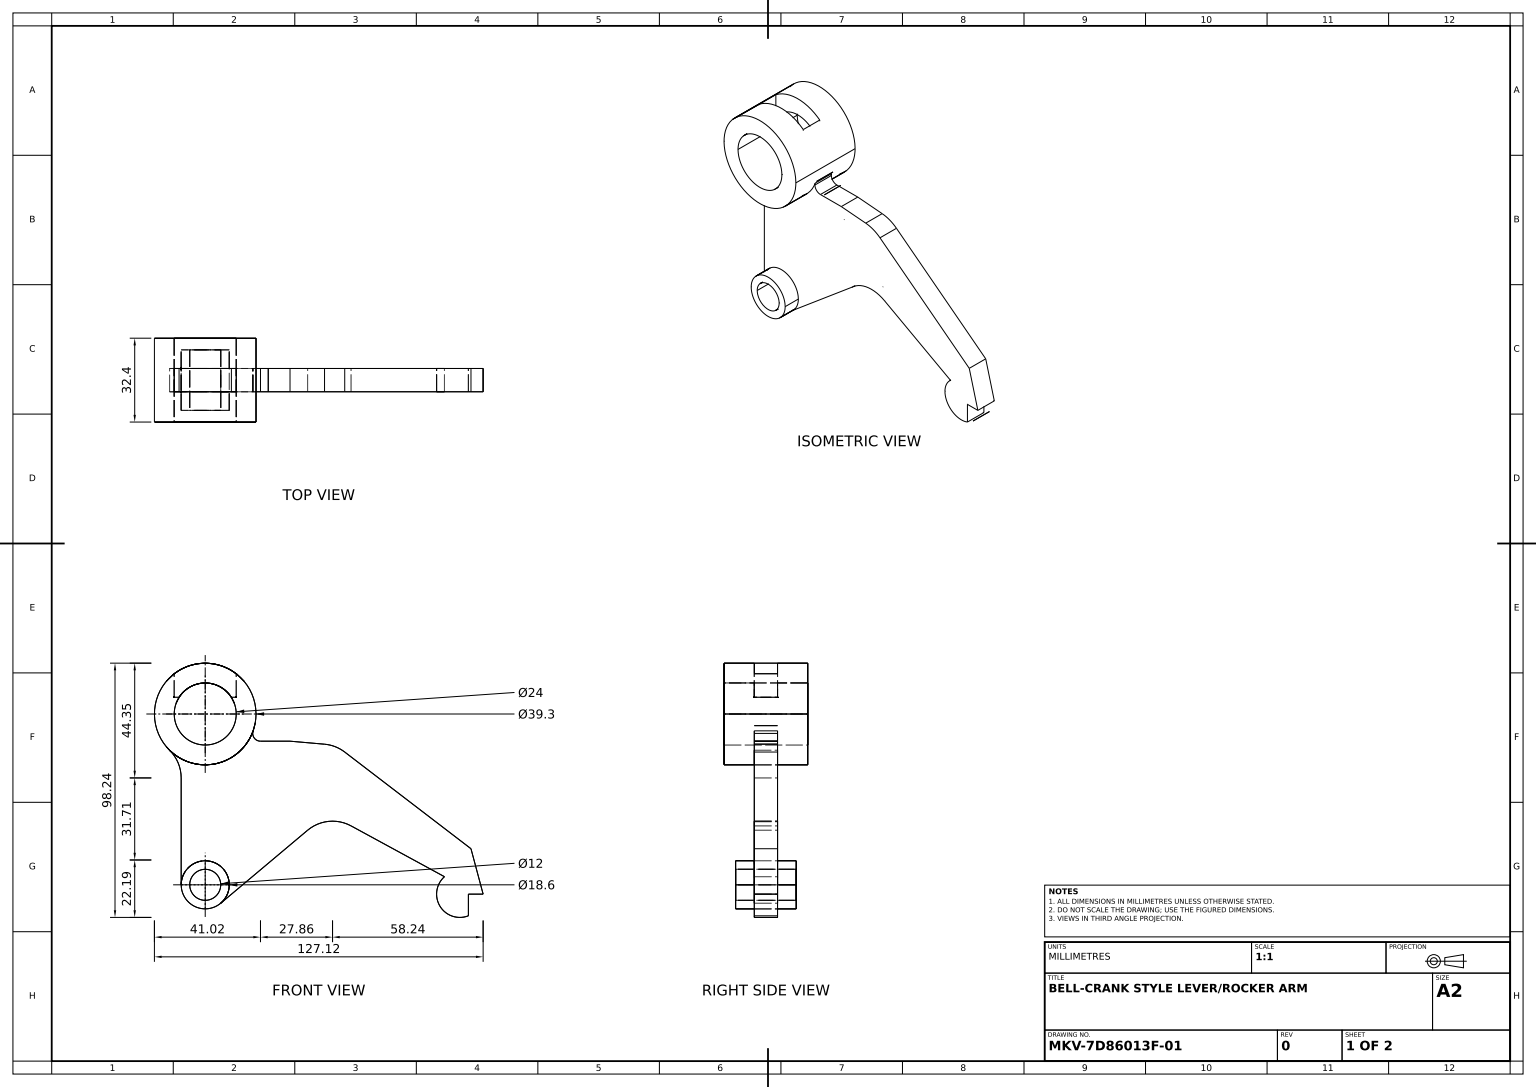
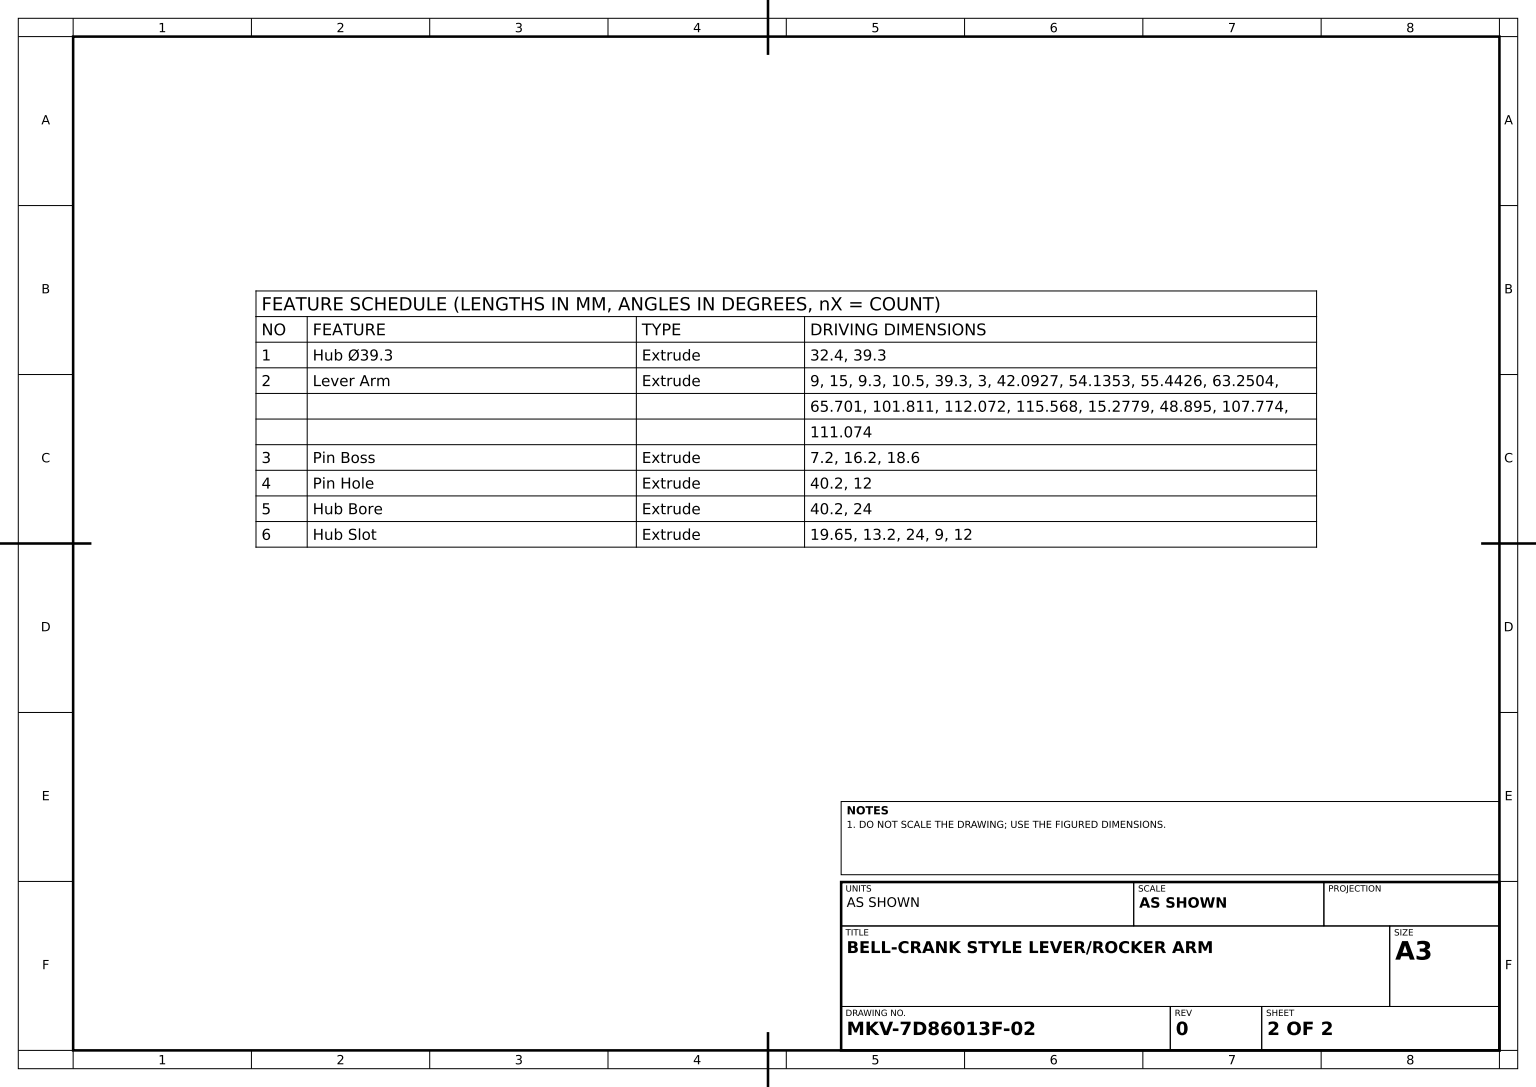
from build123d import *

# Parameters (mm, degrees)
HUB_SKETCH_R        = 19.65
HUB_39_3_DEPTH      = 16.2
LEVER_ARM_DEPTH     = 4.5
PIN_BOSS_DEPTH      = 7.2
PIN_BOSS_DEPTH_BACK = 16.2
PIN_BOSS_SKETCH_R   = 9.3
PIN_HOLE_SKETCH_R   = 6
PIN_HOLE_DEPTH      = 40.2
HUB_BORE_SKETCH_R   = 12
HUB_BORE_DEPTH      = 40.2
HUB_SLOT_DEPTH      = 13.2


with BuildPart() as part:
    # Hub Sketch → Hub Ø39.3 (new, symmetric)
    with BuildSketch(Plane.XY):
        Circle(HUB_SKETCH_R)
    extrude(amount=HUB_39_3_DEPTH, both=True)

    # Lever Arm Sketch → Lever Arm (add, symmetric)
    with BuildSketch(Plane.XY):
        with BuildLine():
            Line((-9.3, -24.700860309), (-9.3, -66))
            ThreePointArc((-9.3, -66), (-3.930349834, -74.428662419), (5.97792477, -73.124213321))
            Line((5.97792477, -73.124213321), (39.595019689, -44.916121374))
            ThreePointArc((39.595019689, -44.916121374), (47.737857787, -41.481873588), (56.401006262, -43.228220821))
            Line((56.401006262, -43.228220821), (92.511102657, -62.858500278))
            ThreePointArc((92.511102657, -62.858500278), (90.79997011, -74.302591391), (101.773667668, -77.973171442))
            Line((101.773667668, -77.973171442), (101.773667668, -69.6))
            Line((101.773667668, -69.6), (107.473667668, -69.6))
            Line((107.473667668, -69.6), (106.267896302, -65.1))
            Line((106.267896302, -65.1), (102.772365267, -52.054500578))
            Line((102.772365267, -52.054500578), (53.950427648, -14.698104885))
            ThreePointArc((53.950427648, -14.698104885), (50.262300823, -12.627051677), (46.142629433, -11.667964344))
            Line((46.142629433, -11.667964344), (32.79273589, -10.5))
            Line((32.79273589, -10.5), (21.372236663, -10.5))
            ThreePointArc((21.372236663, -10.5), (18.924775484, -9.234916071), (18.541476841, -6.506622517))
            ThreePointArc((18.541476841, -6.506622517), (4.442271, -19.141283352), (-13.780519481, -14.007847188))
            ThreePointArc((-13.780519481, -14.007847188), (-10.465401925, -18.903973549), (-9.3, -24.700860309))
        make_face()
    extrude(amount=LEVER_ARM_DEPTH, both=True)

    # Pin Boss Sketch → Pin Boss (add, two sides: drawn at the far end of the back side and taken through both)
    with BuildSketch(Plane.XY.offset(4.5).offset(-PIN_BOSS_DEPTH_BACK)):
        with Locations((0, -66)):
            Circle(PIN_BOSS_SKETCH_R)
    extrude(amount=PIN_BOSS_DEPTH + PIN_BOSS_DEPTH_BACK)

    # Pin Hole Sketch → Pin Hole (cut)
    with BuildSketch(Plane.XY.offset(11.7)):
        with Locations((0, -66)):
            Circle(PIN_HOLE_SKETCH_R)
    extrude(amount=-PIN_HOLE_DEPTH, mode=Mode.SUBTRACT)

    # Hub Bore Sketch → Hub Bore (cut)
    with BuildSketch(Plane.XY.offset(16.2)):
        Circle(HUB_BORE_SKETCH_R)
    extrude(amount=-HUB_BORE_DEPTH, mode=Mode.SUBTRACT)

    # Hub Slot Sketch → Hub Slot (cut)
    with BuildSketch(Plane(origin=(0, 19.65, 0), x_dir=(1, 0, 0), z_dir=(0, 1, 0))):
        Polygon((-12, 0), (-12, 4.5), (12, 4.5), (12, -4.5), (-12, -4.5), align=None)
    extrude(amount=-HUB_SLOT_DEPTH, mode=Mode.SUBTRACT)


solid = part.part
